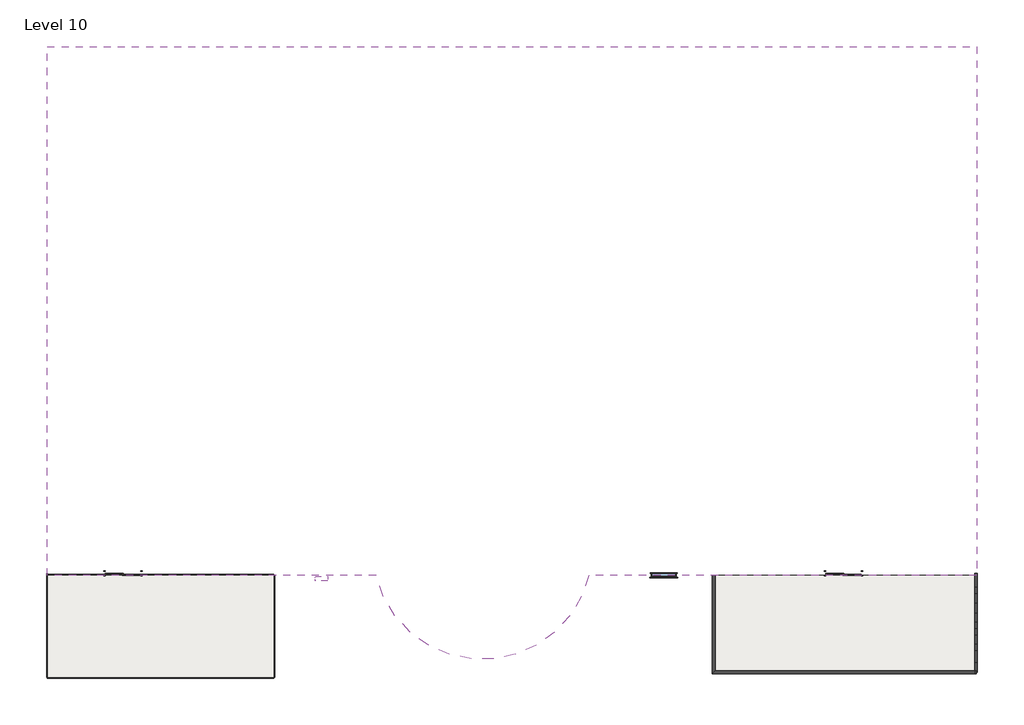
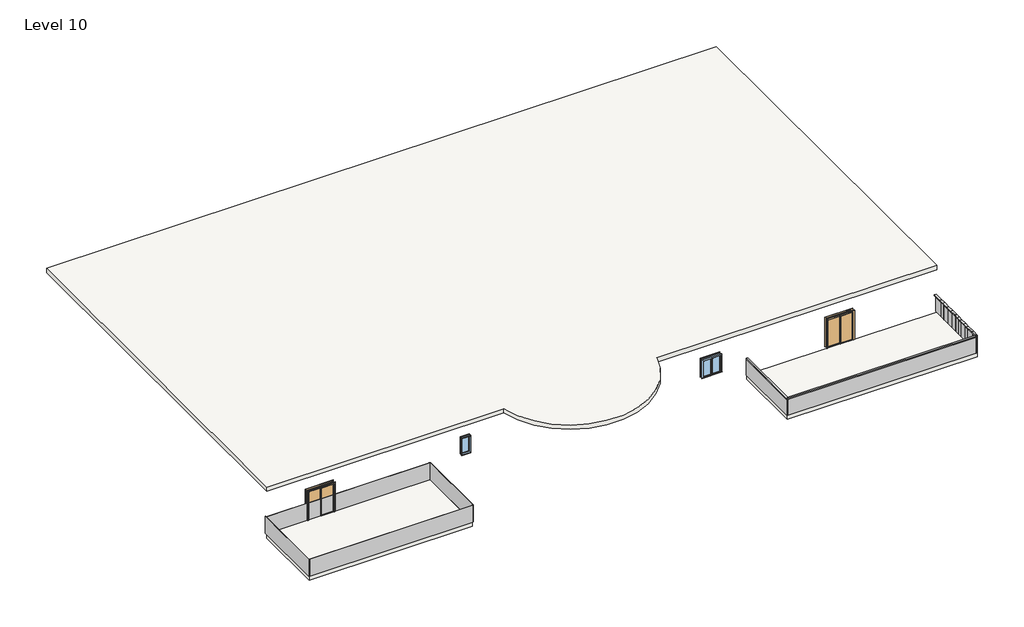
# One storey: 17 plates, 15 members, 3 slabs, 2 doors, 2 windows.
"""IFC4 building model written with IfcOpenShell, lengths in millimetres."""

from ifc_helpers import new_model, si_unit, point, frame, frame_2d, origin, place, context, project, spatial, polyline, circle_curve, trimmed, segment, composite_curve, outline, extrude, transform, mapped, element, save
from components import door_076b30e0, member_75074519, member_47bfaf8a, member_7096a90e, member_15823cb3, member_b46abd34, member_1723abb6, member_b2f14f99, member_19e7b172, member_3c3dc66a, member_aaec729c, system_panel_glazed_7af1c9c3, system_panel_glazed_a18a7e0a, system_panel_glazed_c3939aa2, system_panel_glazed_eef57662, system_panel_glazed_c82e1c3c, system_panel_glazed_c4418efd, system_panel_glazed_1fa29e7b, system_panel_glazed_3daf8e53, system_panel_glazed_710bc1bd, system_panel_glazed_b96adab1, system_panel_glazed_d59597fa, system_panel_glazed_89838f9e, window_0862ab64, window_80bd9af0

model = new_model("IFC4")

# Units and contexts
model_context = context("Model", 3, world=origin())
ifc_project = project(units=[si_unit("LENGTHUNIT", "METRE", prefix="MILLI")], contexts=[model_context])

# Site, building, storey
site = spatial("IfcSite", under=ifc_project)
building = spatial("IfcBuilding", under=site)
storey = spatial("IfcBuildingStorey", under=building, Name="Level 10", Elevation=16459.2)

# Doors
placement = place(None, origin())
door_shape = door_076b30e0(model_context)
element("IfcDoor", 1, ObjectType="Door-Double-Sliding : 68\" x 80\"", at=placement, inside=storey, context=model_context, shape_type="MappedRepresentation", body=[
    mapped(door_shape, transform((-16140.785279, -12227.7237084, 16459.2), x_axis=(-1.0, 0.0, 0.0), y_axis=(0.0, -1.0, 0.0), z_axis=(0.0, 0.0, 1.0))),
])
element("IfcDoor", 2, ObjectType="Door-Double-Sliding : 68\" x 80\"", at=placement, inside=storey, context=model_context, shape_type="MappedRepresentation", body=[
    mapped(door_shape, transform((18987.414721, -12227.7237084, 16459.2), x_axis=(-1.0, 0.0, 0.0), y_axis=(0.0, -1.0, 0.0), z_axis=(0.0, 0.0, 1.0))),
])

# Members
member_shape = member_75074519(model_context)
element("IfcMember", 3, ObjectType="Rectangular Mullion : 2.5\" x 5\" rectangular", at=placement, inside=storey, context=model_context, shape_type="MappedRepresentation", body=[
    mapped(member_shape, transform((25466.4583701, -17186.0208035, 17678.4), x_axis=(1.0, 0.0, 0.0), y_axis=(0.0, 1.0, 0.0), z_axis=(0.0, 0.0, 1.0))),
])
member_2_shape = member_47bfaf8a(model_context)
element("IfcMember", 4, ObjectType="Rectangular Mullion : 2.5\" x 5\" rectangular", at=placement, inside=storey, context=model_context, shape_type="MappedRepresentation", body=[
    mapped(member_2_shape, transform((25466.4583701, -16728.8208035, 17678.4), x_axis=(0.0, 0.0, 1.0), y_axis=(-1.0, 0.0, 0.0), z_axis=(0.0, -1.0, 0.0))),
])
element("IfcMember", 5, ObjectType="Rectangular Mullion : 2.5\" x 5\" rectangular", at=placement, inside=storey, context=model_context, shape_type="MappedRepresentation", body=[
    mapped(member_shape, transform((25466.4583701, -17186.0208035, 16459.2), x_axis=(0.0, -1.0, 0.0), y_axis=(-1.0, 0.0, 0.0), z_axis=(0.0, 0.0, -1.0))),
])
member_3_shape = member_7096a90e(model_context)
element("IfcMember", 6, ObjectType="Rectangular Mullion : 2.5\" x 5\" rectangular", at=placement, inside=storey, context=model_context, shape_type="MappedRepresentation", body=[
    mapped(member_3_shape, transform((25466.4583701, -17122.5208035, 17678.4), x_axis=(0.0, 0.0, 1.0), y_axis=(-1.0, 0.0, 0.0), z_axis=(0.0, -1.0, 0.0))),
])
member_4_shape = member_15823cb3(model_context)
element("IfcMember", 7, ObjectType="Rectangular Mullion : 2.5\" x 5\" rectangular", at=placement, inside=storey, context=model_context, shape_type="MappedRepresentation", body=[
    mapped(member_4_shape, transform((25466.4583701, -14290.4208035, 17678.4), x_axis=(0.0, 0.0, 1.0), y_axis=(-1.0, 0.0, 0.0), z_axis=(0.0, -1.0, 0.0))),
])
element("IfcMember", 8, ObjectType="Rectangular Mullion : 2.5\" x 5\" rectangular", at=placement, inside=storey, context=model_context, shape_type="MappedRepresentation", body=[
    mapped(member_4_shape, transform((25466.4583701, -14747.6208035, 17678.4), x_axis=(0.0, 0.0, 1.0), y_axis=(-1.0, 0.0, 0.0), z_axis=(0.0, -1.0, 0.0))),
])
element("IfcMember", 9, ObjectType="Rectangular Mullion : 2.5\" x 5\" rectangular", at=placement, inside=storey, context=model_context, shape_type="MappedRepresentation", body=[
    mapped(member_4_shape, transform((25466.4583701, -15814.4208035, 17678.4), x_axis=(0.0, 0.0, 1.0), y_axis=(-1.0, 0.0, 0.0), z_axis=(0.0, -1.0, 0.0))),
])
member_5_shape = member_b46abd34(model_context)
element("IfcMember", 10, ObjectType="Rectangular Mullion : 2.5\" x 5\" rectangular", at=placement, inside=storey, context=model_context, shape_type="MappedRepresentation", body=[
    mapped(member_5_shape, transform((12667.5594464, -17186.0208035, 17678.4), x_axis=(0.0, 0.0, 1.0), y_axis=(0.0, 1.0, 0.0), z_axis=(-1.0, 0.0, 0.0))),
])
member_6_shape = member_1723abb6(model_context)
element("IfcMember", 11, ObjectType="Rectangular Mullion : 2.5\" x 5\" rectangular", at=placement, inside=storey, context=model_context, shape_type="MappedRepresentation", body=[
    mapped(member_6_shape, transform((25466.4583701, -13011.8335284, 17678.4), x_axis=(0.0, 0.0, 1.0), y_axis=(-1.0, 0.0, 0.0), z_axis=(0.0, -1.0, 0.0))),
])
member_7_shape = member_b2f14f99(model_context)
element("IfcMember", 12, ObjectType="Rectangular Mullion : 2.5\" x 5\" rectangular", at=placement, inside=storey, context=model_context, shape_type="MappedRepresentation", body=[
    mapped(member_7_shape, transform((25466.4583701, -13340.3884385, 17678.4), x_axis=(0.0, 0.0, 1.0), y_axis=(-1.0, 0.0, 0.0), z_axis=(0.0, -1.0, 0.0))),
])
member_8_shape = member_19e7b172(model_context)
element("IfcMember", 13, ObjectType="Rectangular Mullion : 2.5\" x 5\" rectangular", at=placement, inside=storey, context=model_context, shape_type="MappedRepresentation", body=[
    mapped(member_8_shape, transform((25466.4583701, -13833.2208035, 17678.4), x_axis=(0.0, 0.0, 1.0), y_axis=(-1.0, 0.0, 0.0), z_axis=(0.0, -1.0, 0.0))),
])
member_9_shape = member_3c3dc66a(model_context)
element("IfcMember", 14, ObjectType="Rectangular Mullion : 2.5\" x 5\" rectangular", at=placement, inside=storey, context=model_context, shape_type="MappedRepresentation", body=[
    mapped(member_9_shape, transform((25466.4583701, -15052.4208035, 17678.4), x_axis=(0.0, 0.0, 1.0), y_axis=(-1.0, 0.0, 0.0), z_axis=(0.0, -1.0, 0.0))),
])
element("IfcMember", 15, ObjectType="Rectangular Mullion : 2.5\" x 5\" rectangular", at=placement, inside=storey, context=model_context, shape_type="MappedRepresentation", body=[
    mapped(member_9_shape, transform((25466.4583701, -15357.2208035, 17678.4), x_axis=(0.0, 0.0, 1.0), y_axis=(-1.0, 0.0, 0.0), z_axis=(0.0, -1.0, 0.0))),
])
element("IfcMember", 16, ObjectType="Rectangular Mullion : 2.5\" x 5\" rectangular", at=placement, inside=storey, context=model_context, shape_type="MappedRepresentation", body=[
    mapped(member_9_shape, transform((25466.4583701, -16119.2208035, 17678.4), x_axis=(0.0, 0.0, 1.0), y_axis=(-1.0, 0.0, 0.0), z_axis=(0.0, -1.0, 0.0))),
])
member_10_shape = member_aaec729c(model_context)
element("IfcMember", 17, ObjectType="Rectangular Mullion : 2.5\" x 5\" rectangular", at=placement, inside=storey, context=model_context, shape_type="MappedRepresentation", body=[
    mapped(member_10_shape, transform((12667.5594464, -12456.3237084, 17678.4), x_axis=(0.0, 0.0, 1.0), y_axis=(1.0, 0.0, 0.0), z_axis=(0.0, 1.0, 0.0))),
])

# Plates
system_panel_glazed_shape = system_panel_glazed_7af1c9c3(model_context)
element("IfcPlate", 18, ObjectType="System Panel : Glazed", at=placement, inside=storey, context=model_context, shape_type="MappedRepresentation", body=[
    mapped(system_panel_glazed_shape, transform((25466.4583701, -16424.0208035, 16459.2), x_axis=(0.0, -1.0, 0.0), y_axis=(1.0, 0.0, 0.0), z_axis=(0.0, 0.0, 1.0))),
])
system_panel_glazed_2_shape = system_panel_glazed_a18a7e0a(model_context)
element("IfcPlate", 19, ObjectType="System Panel : Glazed", at=placement, inside=storey, context=model_context, shape_type="MappedRepresentation", body=[
    mapped(system_panel_glazed_2_shape, transform((25466.4583701, -15585.8208035, 16459.2), x_axis=(0.0, -1.0, 0.0), y_axis=(1.0, 0.0, 0.0), z_axis=(0.0, 0.0, 1.0))),
])
element("IfcPlate", 20, ObjectType="System Panel : Glazed", at=placement, inside=storey, context=model_context, shape_type="MappedRepresentation", body=[
    mapped(system_panel_glazed_2_shape, transform((25466.4583701, -14519.0208035, 16459.2), x_axis=(0.0, -1.0, 0.0), y_axis=(1.0, 0.0, 0.0), z_axis=(0.0, 0.0, 1.0))),
])
element("IfcPlate", 21, ObjectType="System Panel : Glazed", at=placement, inside=storey, context=model_context, shape_type="MappedRepresentation", body=[
    mapped(system_panel_glazed_2_shape, transform((25466.4583701, -14061.8208035, 16459.2), x_axis=(0.0, -1.0, 0.0), y_axis=(1.0, 0.0, 0.0), z_axis=(0.0, 0.0, 1.0))),
])
system_panel_glazed_3_shape = system_panel_glazed_c3939aa2(model_context)
element("IfcPlate", 22, ObjectType="System Panel : Glazed", at=placement, inside=storey, context=model_context, shape_type="MappedRepresentation", body=[
    mapped(system_panel_glazed_3_shape, transform((25466.4583701, -16925.6708035, 16459.2), x_axis=(0.0, -1.0, 0.0), y_axis=(1.0, 0.0, 0.0), z_axis=(0.0, 0.0, 1.0))),
])
system_panel_glazed_4_shape = system_panel_glazed_eef57662(model_context)
element("IfcPlate", 23, ObjectType="System Panel : Glazed", at=placement, inside=storey, context=model_context, shape_type="MappedRepresentation", body=[
    mapped(system_panel_glazed_4_shape, transform((12667.5594464, -14821.1722559, 16459.2), x_axis=(0.0, 1.0, 0.0), y_axis=(-1.0, 0.0, 0.0), z_axis=(0.0, 0.0, 1.0))),
])
system_panel_glazed_5_shape = system_panel_glazed_c82e1c3c(model_context)
element("IfcPlate", 24, ObjectType="System Panel : Glazed", at=placement, inside=storey, context=model_context, shape_type="MappedRepresentation", body=[
    mapped(system_panel_glazed_5_shape, transform((19035.2589083, -17186.0208035, 16459.2), x_axis=(-1.0, 0.0, 0.0), y_axis=(0.0, -1.0, 0.0), z_axis=(0.0, 0.0, 1.0))),
])
system_panel_glazed_6_shape = system_panel_glazed_c4418efd(model_context)
element("IfcPlate", 25, ObjectType="System Panel : Glazed", at=placement, inside=storey, context=model_context, shape_type="MappedRepresentation", body=[
    mapped(system_panel_glazed_6_shape, transform((25466.4583701, -12683.2786184, 16459.2), x_axis=(0.0, -1.0, 0.0), y_axis=(1.0, 0.0, 0.0), z_axis=(0.0, 0.0, 1.0))),
])
system_panel_glazed_7_shape = system_panel_glazed_1fa29e7b(model_context)
element("IfcPlate", 26, ObjectType="System Panel : Glazed", at=placement, inside=storey, context=model_context, shape_type="MappedRepresentation", body=[
    mapped(system_panel_glazed_7_shape, transform((25466.4583701, -15966.8208035, 16459.2), x_axis=(0.0, -1.0, 0.0), y_axis=(1.0, 0.0, 0.0), z_axis=(0.0, 0.0, 1.0))),
])
element("IfcPlate", 27, ObjectType="System Panel : Glazed", at=placement, inside=storey, context=model_context, shape_type="MappedRepresentation", body=[
    mapped(system_panel_glazed_7_shape, transform((25466.4583701, -15204.8208035, 16459.2), x_axis=(0.0, -1.0, 0.0), y_axis=(1.0, 0.0, 0.0), z_axis=(0.0, 0.0, 1.0))),
])
element("IfcPlate", 28, ObjectType="System Panel : Glazed", at=placement, inside=storey, context=model_context, shape_type="MappedRepresentation", body=[
    mapped(system_panel_glazed_7_shape, transform((25466.4583701, -14900.0208035, 16459.2), x_axis=(0.0, -1.0, 0.0), y_axis=(1.0, 0.0, 0.0), z_axis=(0.0, 0.0, 1.0))),
])
system_panel_glazed_8_shape = system_panel_glazed_3daf8e53(model_context)
element("IfcPlate", 29, ObjectType="System Panel : Glazed", at=placement, inside=storey, context=model_context, shape_type="MappedRepresentation", body=[
    mapped(system_panel_glazed_8_shape, transform((25466.4583701, -13586.804621, 16459.2), x_axis=(0.0, -1.0, 0.0), y_axis=(1.0, 0.0, 0.0), z_axis=(0.0, 0.0, 1.0))),
])
system_panel_glazed_9_shape = system_panel_glazed_710bc1bd(model_context)
element("IfcPlate", 30, ObjectType="System Panel : Glazed", at=placement, inside=storey, context=model_context, shape_type="MappedRepresentation", body=[
    mapped(system_panel_glazed_9_shape, transform((25466.4583701, -13176.1109835, 16459.2), x_axis=(0.0, -1.0, 0.0), y_axis=(1.0, 0.0, 0.0), z_axis=(0.0, 0.0, 1.0))),
])
system_panel_glazed_10_shape = system_panel_glazed_b96adab1(model_context)
element("IfcPlate", 31, ObjectType="System Panel : Glazed", at=placement, inside=storey, context=model_context, shape_type="MappedRepresentation", body=[
    mapped(system_panel_glazed_10_shape, transform((-14302.7926538, -12456.3237084, 16459.2), x_axis=(1.0, 0.0, 0.0), y_axis=(0.0, 1.0, 0.0), z_axis=(0.0, 0.0, 1.0))),
])
element("IfcPlate", 32, ObjectType="System Panel : Glazed", at=placement, inside=storey, context=model_context, shape_type="MappedRepresentation", body=[
    mapped(system_panel_glazed_10_shape, transform((-14302.7926538, -17427.6878561, 16459.2), x_axis=(-1.0, 0.0, 0.0), y_axis=(0.0, -1.0, 0.0), z_axis=(0.0, 0.0, 1.0))),
])
system_panel_glazed_11_shape = system_panel_glazed_d59597fa(model_context)
element("IfcPlate", 33, ObjectType="System Panel : Glazed", at=placement, inside=storey, context=model_context, shape_type="MappedRepresentation", body=[
    mapped(system_panel_glazed_11_shape, transform((-8781.8000285, -14942.0057823, 16459.2), x_axis=(0.0, -1.0, 0.0), y_axis=(1.0, 0.0, 0.0), z_axis=(0.0, 0.0, 1.0))),
])
system_panel_glazed_12_shape = system_panel_glazed_89838f9e(model_context)
element("IfcPlate", 34, ObjectType="System Panel : Glazed", at=placement, inside=storey, context=model_context, shape_type="MappedRepresentation", body=[
    mapped(system_panel_glazed_12_shape, transform((-19823.785279, -14891.2057823, 16459.2), x_axis=(0.0, 1.0, 0.0), y_axis=(-1.0, 0.0, 0.0), z_axis=(0.0, 0.0, 1.0))),
])

# Slabs
element("IfcSlab", 35, ObjectType="Generic - 12\"", at=placement, inside=storey, context=model_context, shape_type="SweptSolid", body=[
    extrude(outline(composite_curve([segment(polyline([(25489.814721, 13350.0762916), (25489.814721, -12456.3237084), (6571.5594464, -12456.3237084)]), True, "CONTINUOUS"), segment(trimmed(circle_curve(frame_2d((1385.214721, -11225.6906671)), 5330.3498284), [point((6571.5594464, -12456.3237084))], [point((-3801.1300045, -12456.3237084))], False, "CARTESIAN"), True, "CONTINUOUS"), segment(polyline([(-3801.1300045, -12456.3237084), (-19823.785279, -12456.3237084), (-19823.785279, 13350.0762916), (25489.814721, 13350.0762916)]), True, "CONTINUOUS")], self_intersect=False)), frame((0.0, 0.0, 19506.9268686), z_axis=(0.0, 0.0, 1.0), x_axis=(1.0, 0.0, 0.0)), (0.0, 0.0, 1.0), 304.8),
])
element("IfcSlab", 36, ObjectType="Generic - 12\"", at=placement, inside=storey, context=model_context, shape_type="SweptSolid", body=[
    extrude(outline(polyline([(25489.814721, -12456.3237084), (25489.814721, -17203.521287), (12667.5594464, -17203.521287), (12667.5594464, -12456.3237084), (25489.814721, -12456.3237084)])), frame((0.0, 0.0, 16154.4), z_axis=(0.0, 0.0, 1.0), x_axis=(1.0, 0.0, 0.0)), (0.0, 0.0, 1.0), 304.8),
])
element("IfcSlab", 37, ObjectType="Generic - 12\"", at=placement, inside=storey, context=model_context, shape_type="SweptSolid", body=[
    extrude(outline(polyline([(-8781.8000285, -12456.3237084), (-8781.8000285, -17427.6878561), (-19823.785279, -17427.6878561), (-19823.785279, -12456.3237084), (-8781.8000285, -12456.3237084)])), frame((0.0, 0.0, 16154.4), z_axis=(0.0, 0.0, 1.0), x_axis=(1.0, 0.0, 0.0)), (0.0, 0.0, 1.0), 304.8),
])

# Windows
window_shape = window_0862ab64(model_context)
element("IfcWindow", 38, ObjectType="Casement Dbl with Trim : 48\" x 48\"", at=placement, inside=storey, context=model_context, shape_type="MappedRepresentation", body=[
    mapped(window_shape, transform((10229.1594464, -12437.2737084, 16459.2), x_axis=(-1.0, 0.0, 0.0), y_axis=(0.0, -1.0, 0.0), z_axis=(0.0, 0.0, 1.0))),
])
window_2_shape = window_80bd9af0(model_context)
element("IfcWindow", 39, ObjectType="Fixed : 24\" x 48\"", at=placement, inside=storey, context=model_context, shape_type="MappedRepresentation", body=[
    mapped(window_2_shape, transform((-6425.285279, -12617.2007309, 16745.1066858), x_axis=(1.0, 0.0, 0.0), y_axis=(0.0, 1.0, 0.0), z_axis=(0.0, 0.0, 1.0))),
])

save(model, "model.ifc")

# Revit data of these elements
# Type "Door-Double-Sliding : 68\" x 80\""
#   Type Mark = "10"
#   Construction Type Id = "opn-d45"
#   Assembly Code = "C1020"
#   Analytic Construction = "Wood frame, double glass door "
#   Thickness = 0' - 2"
#   Thermal Resistance (R) = 1.8150 (h·ft²·°F)/BTU
#   Heat Transfer Coefficient (U) = 0.5510 BTU/(h·ft²·°F)
#   Height = 6' - 8"
#   Rail Width = 0' - 2"
#   Stiles = 0' - 2"
#   Trim Projection Ext = 0' - 1"
#   Trim Projection Int = 0' - 1"
#   Trim Width = 0' - 3"
#   Width = 5' - 8"
#   Define Thermal Properties by = 1
#   Glazing = Glass
#   Panel Material = Wood - Birch - Solid Stained Light Low Gloss
#   Trim Material = Paint - Sienna
#   Visual Light Transmittance = 0
#   Solar Heat Gain Coefficient = 0
#   Function = (empty or 0)
#   Wall Closure = (empty or 0)
# Type "Rectangular Mullion : 2.5\" x 5\" rectangular"
#   built-in parameter 1007304 = 0.416667 (stored number, unit not read)
#   built-in parameter 1007301 = 0.104167 (stored number, unit not read)
#   built-in parameter 1007300 = 0.104167 (stored number, unit not read)
# Type "System Panel : Glazed"
#   Construction Type Id = "GSP4R"
#   Analytic Construction = "1/8 in Pilkington single glazing"
#   Visual Light Transmittance = 0.9
#   Solar Heat Gain Coefficient = 0.86
#   Heat Transfer Coefficient (U) = 1.18115 BTU/(h·ft²·°F)
# Type "Generic - 12\""
#   Assembly Code = "B1010"
#   Function = 0
#   Layers, outside or top first: 1' - 0" no material (function 1)
# Type "Casement Dbl with Trim : 48\" x 48\""
#   Type Mark = "34"
#   Construction Type Id = "GSP4R"
#   Assembly Code = "B2020100"
#   Analytic Construction = "1/8 in Pilkington single glazing"
#   Visual Light Transmittance = 0.9
#   Solar Heat Gain Coefficient = 0.78
#   Heat Transfer Coefficient (U) = 0.6496 BTU/(h·ft²·°F)
#   Height = 4' - 0"
#   Default Sill Height = 3' - 0"
#   Trim Projection - Ext. = 0' - 0 1/2"
#   Trim Projection - Int. = 0' - 0 3/4"
#   Trim Width - Exterior = 0' - 3 1/2"
#   Trim Width - Interior = 0' - 3 1/2"
#   Width = 4' - 0"
#   Window Inset = 0' - 0 3/4"
#   Define Thermal Properties by = 1
#   Glass Pane Material = Glass
#   Sash Material = Sash
#   Trim Exterior Material = Trim
#   Trim Interior Material = Trim
#   Wall Closure = (empty or 0)
# Type "Fixed : 24\" x 48\""
#   Type Mark = "2"
#   Construction Type Id = "GSP4R"
#   Assembly Code = "B2020100"
#   Analytic Construction = "1/8 in Pilkington single glazing"
#   Visual Light Transmittance = 0.9
#   Solar Heat Gain Coefficient = 0.78
#   Heat Transfer Coefficient (U) = 0.6496 BTU/(h·ft²·°F)
#   Height = 4' - 0"
#   Default Sill Height = 3' - 0"
#   Width = 2' - 0"
#   Window Inset = 0' - 0 3/4"
#   Define Thermal Properties by = 1
#   Glass Pane Material = Glass
#   Sash Material = Sash
#   Wall Closure = (empty or 0)
# Elements 1, 2 (IfcDoor, "Door-Double-Sliding : 68\" x 80\"")
#   Phase Created = New Construction
#   Materials on its faces: "Paint - Sienna", "Wood - Birch - Solid Stained Light Low Gloss", "Glass"
# Elements 3, 4, 5, 6, 7, 8, 9, 10, 11, 12, 13, 14, 15, 16, 17 (IfcMember, "Rectangular Mullion : 2.5\" x 5\" rectangular")
#   Phase Created = New Construction
#   Materials on its faces: "Aluminum"
# Elements 18, 19, 20, 21, 22, 23, 24, 25, 26, 27, 28, 29, 30, 31, 32, 33, 34 (IfcPlate, "System Panel : Glazed")
#   Phase Created = New Construction
#   Materials on its faces: "Glass"
# Element 35 (IfcSlab, "Generic - 12\"")
#   Height Offset From Level = 10' - 11.98925"
#   Phase Created = New Construction
#   Materials on its faces: "Default Floor"
# Elements 36, 37 (IfcSlab, "Generic - 12\"")
#   Height Offset From Level = 0' - 0"
#   Phase Created = New Construction
#   Materials on its faces: "Default Floor"
# Element 38 (IfcWindow, "Casement Dbl with Trim : 48\" x 48\"")
#   Mark = "12"
#   Phase Created = New Construction
#   Materials on its faces: "Sash", "Trim", "Glass"
# Element 39 (IfcWindow, "Fixed : 24\" x 48\"")
#   Mark = "80"
#   Phase Created = New Construction
#   Materials on its faces: "Sash", "Glass"
# Materials
#   "Glass": class "Glass", colour RGB 0 128 192, transparency 0.75, Description = "Soda Lime Glass", Cost = 0
#   "Wood - Birch - Solid Stained Light Low Gloss": class "Wood", colour RGB 210 159 95, transparency 0, Cost = 0
#   "Paint - Sienna": colour RGB 118 70 51, transparency 0, Cost = 0
#   "Sash": class "Wood", colour RGB 224 178 126, transparency 0
#   "Trim": class "Wood", colour RGB 224 178 126, transparency 0
#   "Aluminum": class "Metal", colour RGB 247 247 247, transparency 0, Description = "Aluminum 6061", Cost = 0
#   "Default Floor": colour RGB 128 128 128, transparency 0
